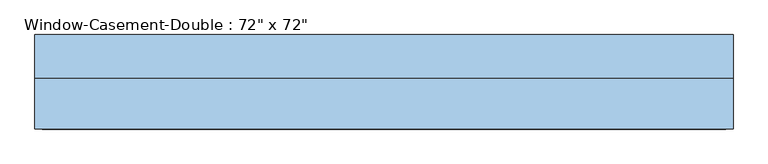
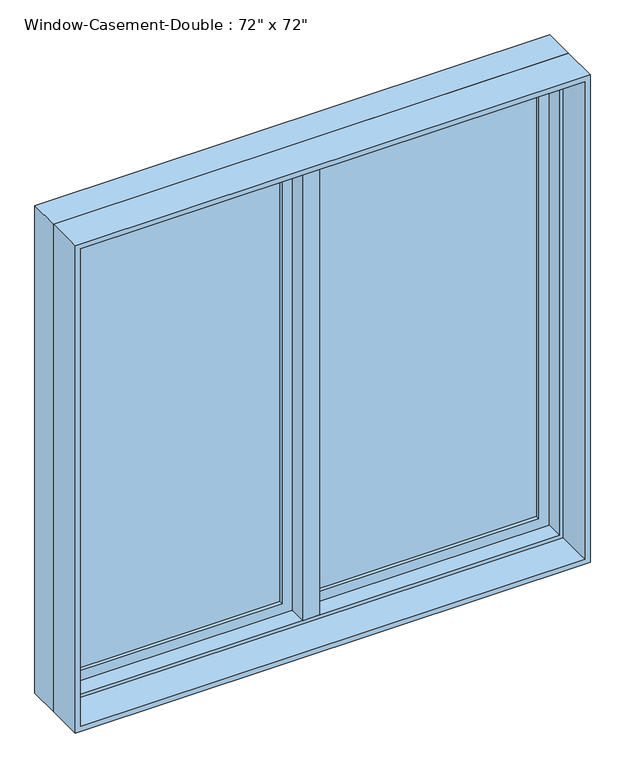
"""IFC4 building model written with IfcOpenShell, lengths in millimetres: window geometry."""

from ifc_helpers import new_model, si_unit, frame, origin, place, context, project, spatial, polyline, outline, extrude, faceted_brep, source, transform, mapped, element, save


def window_ce442eab(model_context):
    return source(origin(), model_context, "Body", "SolidModel", [
        faceted_brep([(9.525, 133.35, 2730.5), (-9.525, 133.35, 2730.5), (-9.525, 82.55, 2730.5), (9.525, 82.55, 2730.5), (9.525, 133.35, 927.1), (9.525, 82.55, 927.1), (-9.525, 82.55, 927.1), (-9.525, 133.35, 927.1), (-9.525, 82.55, 946.15), (-9.525, 82.55, 2711.45), (-30.1625, 82.55, 946.15), (-30.1625, 82.55, 2711.45), (-30.1625, 19.05, 946.15), (-30.1625, 19.05, 2711.45), (30.1625, 19.05, 946.15), (30.1625, 19.05, 2711.45), (30.1625, 82.55, 946.15), (30.1625, 82.55, 2711.45), (9.525, 82.55, 946.15), (9.525, 82.55, 2711.45)], [[[0, 1, 2, 3]], [[4, 5, 6, 7]], [[1, 0, 4, 7]], [[2, 1, 7, 6, 8, 9]], [[9, 8, 10, 11]], [[11, 10, 12, 13]], [[13, 12, 14, 15]], [[15, 14, 16, 17]], [[17, 16, 18, 19]], [[0, 3, 19, 18, 5, 4]], [[18, 8, 6, 5]], [[9, 19, 3, 2]], [[8, 18, 16, 14, 12, 10]], [[19, 9, 11, 13, 15, 17]]]),
        extrude(outline(polyline([(-66.675, 114.3), (-66.675, 107.95), (-844.55, 107.95), (-844.55, 114.3), (-66.675, 114.3)])), frame((0.0, 0.0, 984.25), z_axis=(0.0, 0.0, 1.0), x_axis=(1.0, 0.0, 0.0)), (0.0, 0.0, 1.0), 1689.1),
        extrude(outline(polyline([(-844.55, 95.25), (-844.55, 101.6), (-66.675, 101.6), (-66.675, 95.25), (-844.55, 95.25)])), frame((0.0, 0.0, 984.25), z_axis=(0.0, 0.0, 1.0), x_axis=(1.0, 0.0, 0.0)), (0.0, 0.0, 1.0), 1689.1),
        extrude(outline(polyline([(844.55, 114.3), (844.55, 107.95), (66.675, 107.95), (66.675, 114.3), (844.55, 114.3)])), frame((0.0, 0.0, 984.25), z_axis=(0.0, 0.0, 1.0), x_axis=(1.0, 0.0, 0.0)), (0.0, 0.0, 1.0), 1689.1),
        extrude(outline(polyline([(66.675, 95.25), (66.675, 101.6), (844.55, 101.6), (844.55, 95.25), (66.675, 95.25)])), frame((0.0, 0.0, 984.25), z_axis=(0.0, 0.0, 1.0), x_axis=(1.0, 0.0, 0.0)), (0.0, 0.0, 1.0), 1689.1),
        extrude(outline(polyline([(2730.5, -901.7), (927.1, -901.7), (927.1, -9.525), (2730.5, -9.525), (2730.5, -901.7)]), holes=[polyline([(2673.35, -66.675), (984.25, -66.675), (984.25, -844.55), (2673.35, -844.55), (2673.35, -66.675)])]), frame((0.0, 82.55, 0.0), z_axis=(0.0, 1.0, 0.0), x_axis=(0.0, 0.0, 1.0)), (0.0, 0.0, 1.0), 44.45),
        extrude(outline(polyline([(927.1, 901.7), (2730.5, 901.7), (2730.5, 9.525), (927.1, 9.525), (927.1, 901.7)]), holes=[polyline([(984.25, 66.675), (2673.35, 66.675), (2673.35, 844.55), (984.25, 844.55), (984.25, 66.675)])]), frame((0.0, 82.55, 0.0), z_axis=(0.0, 1.0, 0.0), x_axis=(0.0, 0.0, 1.0)), (0.0, 0.0, 1.0), 44.45),
        extrude(outline(polyline([(2743.2, -914.4), (914.4, -914.4), (914.4, 914.4), (2743.2, 914.4), (2743.2, -914.4)]), holes=[polyline([(2724.15, 895.35), (933.45, 895.35), (933.45, -895.35), (2724.15, -895.35), (2724.15, 895.35)])]), frame((0.0, -114.3, 0.0), z_axis=(0.0, 1.0, 0.0), x_axis=(0.0, 0.0, 1.0)), (0.0, 0.0, 1.0), 133.35),
        faceted_brep([(882.65, 82.55, 2711.45), (882.65, 19.05, 2711.45), (-882.65, 19.05, 2711.45), (-882.65, 82.55, 2711.45), (901.7, 133.35, 2730.5), (901.7, 82.55, 2730.5), (-901.7, 82.55, 2730.5), (-901.7, 133.35, 2730.5), (914.4, 19.05, 2743.2), (914.4, 133.35, 2743.2), (-914.4, 133.35, 2743.2), (-914.4, 19.05, 2743.2), (-882.65, 19.05, 946.15), (-882.65, 82.55, 946.15), (-901.7, 82.55, 927.1), (-901.7, 133.35, 927.1), (-914.4, 133.35, 914.4), (-914.4, 19.05, 914.4), (882.65, 19.05, 946.15), (882.65, 82.55, 946.15), (901.7, 82.55, 927.1), (901.7, 133.35, 927.1), (914.4, 133.35, 914.4), (914.4, 19.05, 914.4)], [[[0, 1, 2, 3]], [[4, 5, 6, 7]], [[8, 9, 10, 11]], [[3, 2, 12, 13]], [[7, 6, 14, 15]], [[11, 10, 16, 17]], [[13, 12, 18, 19]], [[15, 14, 20, 21]], [[17, 16, 22, 23]], [[11, 17, 23, 8], [1, 18, 12, 2]], [[19, 18, 1, 0]], [[5, 20, 14, 6], [3, 13, 19, 0]], [[21, 20, 5, 4]], [[23, 22, 9, 8]], [[9, 22, 16, 10], [7, 15, 21, 4]]]),
    ])


if __name__ == "__main__":
    model = new_model("IFC4")
    model_context = context("Model", 3, world=origin())
    ifc_project = project(units=[si_unit("LENGTHUNIT", "METRE", prefix="MILLI")], contexts=[model_context])
    site = spatial("IfcSite", under=ifc_project)
    building = spatial("IfcBuilding", under=site)
    placement = place(None, origin())
    window_shape = window_ce442eab(model_context)
    element("IfcWindow", 1, ObjectType="Window-Casement-Double : 72\" x 72\"", at=placement, inside=building, context=model_context, shape_type="MappedRepresentation", body=[
        mapped(window_shape, transform((0.0, 0.0, 0.0), x_axis=(1.0, 0.0, 0.0), y_axis=(0.0, 1.0, 0.0), z_axis=(0.0, 0.0, 1.0))),
    ])
    save(model, "model.ifc")

# Revit data of these elements
# Type "Window-Casement-Double : 72\" x 72\""
#   Type Mark = "18"
#   Fire Rating = "0.5h"
#   Assembly Code = "B2020100"
#   Analytic Construction = "Double glazing - domestic"
#   Frame Extension [instance default] = 0' - 0 1/4"
#   Window Inset [instance default] = 0' - 0"
#   Wall Thickness [instance default] = 0' - 6"
#   Interior Wall Closure [instance default] = 0' - 2 1/4"
#   Half Width = 3' - 0"
#   Visual Light Transmittance = 0.81
#   Thermal Resistance (R) = 1.8146 (h·ft²·°F)/BTU
#   Solar Heat Gain Coefficient = 0.76
#   Rough Width = 6' - 0 1/2"
#   Rough Height = 6' - 0 1/2"
#   Height = 6' - 0"
#   Heat Transfer Coefficient (U) = 0.5511 BTU/(h·ft²·°F)
#   Exterior Wall Closure [instance default] = 0' - 1 1/4"
#   Extension Jamb [instance default] = 0' - 2 1/4"
#   Default Sill Height = 3' - 0"
#   Width = 6' - 0"
#   Muntin Visibility = yes
#   Interior Trim Visibility [instance default] = yes
#   Exterior Trim Visibility [instance default] = yes
#   Extension Jamb Visibility [instance default] = yes
#   Interior Trim Material = Wood - Stained
#   Muntin Pattern = Muntin Pattern_2x2 : Muntin Pattern_2x2
#   Interior Trim = Trim-Window-Interior-Flat : Picture Frame
#   Interior Frame Material = Wood - Stained
#   Glass Panel Material = Glass
#   Exterior Trim Material = Clad - White
#   Exterior Trim = Trim-Window-Exterior-Flat : with Sill
#   Exterior Frame Material = Clad - White
#   Wall Closure = (empty or 0)
# Element 1 (IfcWindow, "Window-Casement-Double : 72\" x 72\"")
#   Wall Thickness = 0' - 9"
#   Extension Jamb = 0' - 5 1/4"
#   Materials on its faces: "Wood - Stained", "Glass", "Clad - White"
# Materials
#   "Wood - Stained": class "Wood", colour RGB 224 178 126, transparency 0, Cost = 0
#   "Glass": class "Glass", colour RGB 0 128 192, transparency 0.75, Description = "Soda Lime Glass", Cost = 0
#   "Clad - White": class "Wood", colour RGB 242 242 238, transparency 0, Cost = 0
